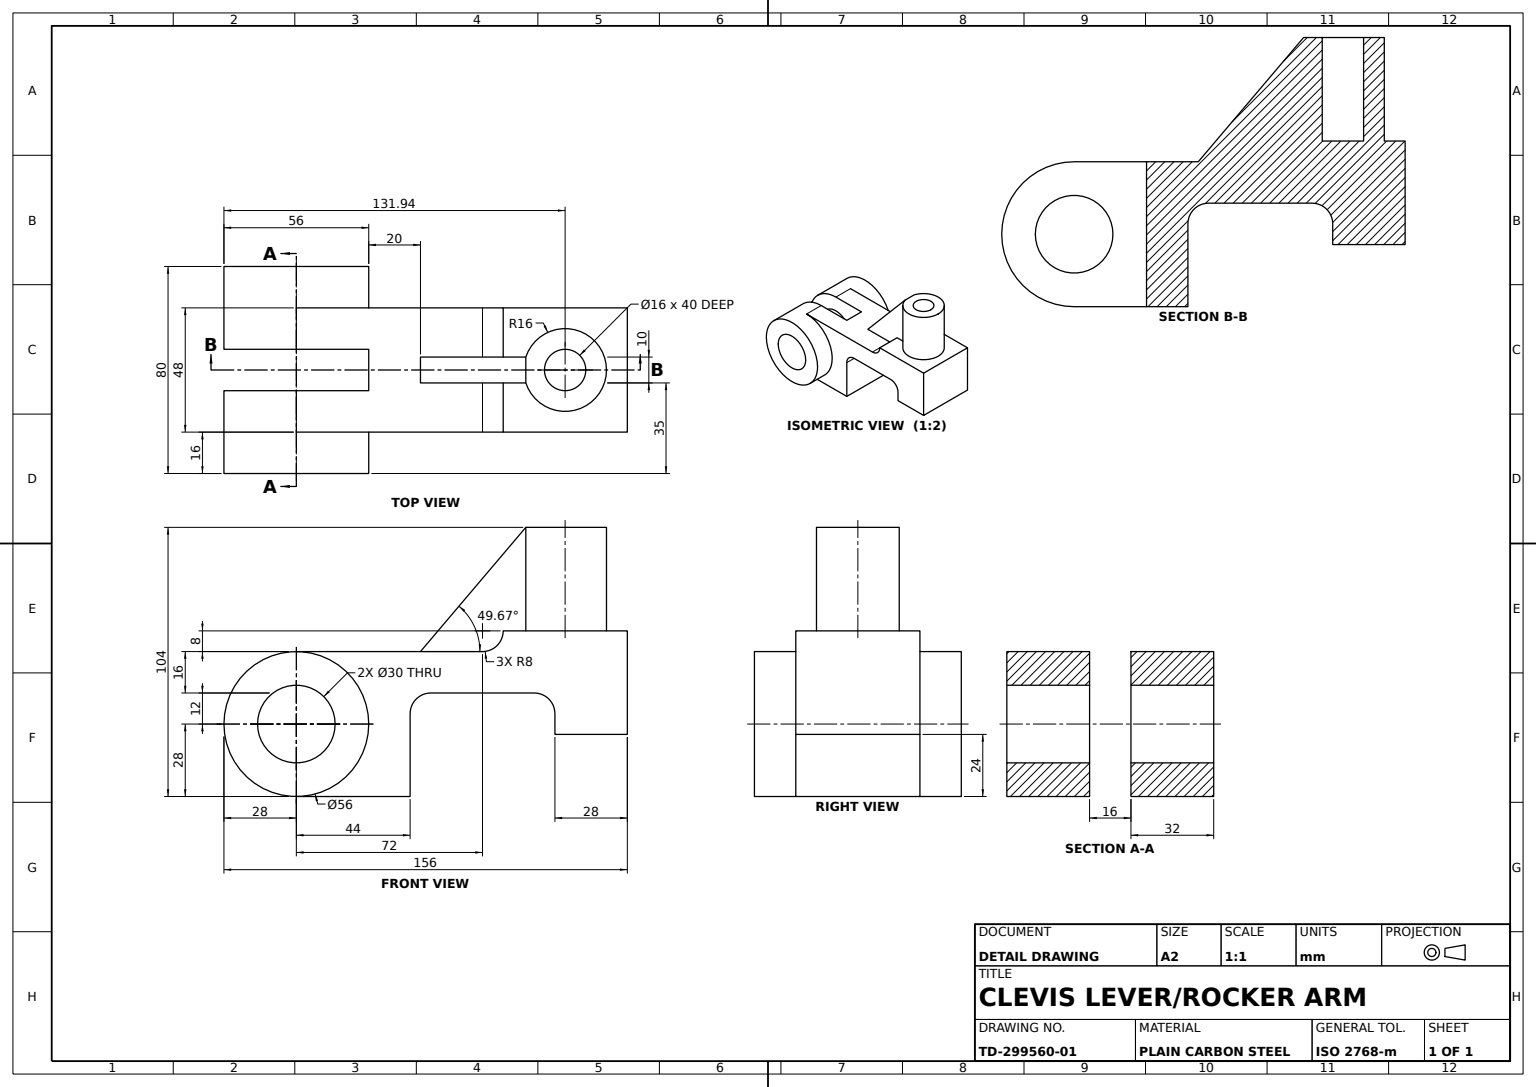
from build123d import *

# Parameters (mm, degrees)
PIVOT_HUB_SKETCH_R            = 28
PIVOT_HUB_SKETCH_R_2          = 15
PIVOT_HUB_56_BORE_30_DEPTH    = 40
LINK_ARM_DEPTH                = 24
FORK_SLOT_SKETCH_W            = 63.247521784
FORK_SLOT_SKETCH_H            = 16
FORK_SLOT_16_DEPTH            = 146.327216997
UPRIGHT_BOSS_SKETCH_R         = 16
UPRIGHT_BOSS_SKETCH_R_2       = 8
UPRIGHT_BOSS_32_BORE_16_DEPTH = 40
JUNCTION_PAD_REACH            = 171.706
TRIANGULAR_RELIEF_CUT_DEPTH   = 10


with BuildPart() as part:
    # Pivot Hub Sketch → Pivot Hub Ø56 Bore Ø30 (new, symmetric)
    with BuildSketch(Plane.XY):
        Circle(PIVOT_HUB_SKETCH_R)
        Circle(PIVOT_HUB_SKETCH_R_2, mode=Mode.SUBTRACT)
    extrude(amount=PIVOT_HUB_56_BORE_30_DEPTH, both=True)

    # Link Arm Profile → Link Arm (add, symmetric)
    with BuildSketch(Plane.XY):
        with BuildLine():
            Line((0, 28), (72, 28))
            ThreePointArc((72, 28), (77.656854249, 30.343145751), (80, 36))
            Line((80, 36), (128, 36))
            Line((128, 36), (128, -4))
            Line((128, -4), (100, -4))
            Line((100, -4), (100, 4))
            ThreePointArc((100, 4), (97.656854249, 9.656854249), (92, 12))
            Line((92, 12), (52, 12))
            ThreePointArc((52, 12), (46.343145751, 9.656854249), (44, 4))
            Line((44, 4), (44, -28))
            Line((44, -28), (0, -28))
            ThreePointArc((0, -28), (28, 0), (0, 28))
        make_face()
    extrude(amount=LINK_ARM_DEPTH, both=True)

    # Fork Slot Sketch → Fork Slot 16 (cut, through all)
    with BuildSketch(Plane(origin=(0, 28, 0), x_dir=(1, 0, 0), z_dir=(0, 1, 0))):
        with Locations((-3.623760892, 0)):
            Rectangle(FORK_SLOT_SKETCH_W, FORK_SLOT_SKETCH_H)
    extrude(amount=-FORK_SLOT_16_DEPTH, mode=Mode.SUBTRACT)

    # Upright Boss Sketch → Upright Boss Ø32 Bore Ø16 (add)
    with BuildSketch(Plane(origin=(0, 36, 0), x_dir=(1, 0, 0), z_dir=(0, 1, 0))):
        with Locations((103.942410132, 0)):
            Circle(UPRIGHT_BOSS_SKETCH_R)
        with Locations(Location((103.942410132, 0, 0), (0, 0, 180))):
            Circle(UPRIGHT_BOSS_SKETCH_R_2, mode=Mode.SUBTRACT)
    extrude(amount=UPRIGHT_BOSS_32_BORE_16_DEPTH)

    # Junction Pad Sketch → Junction Pad (add, up to next)
    with BuildSketch(Plane(origin=(0, 76, 0), x_dir=(1, 0, 0), z_dir=(0, 1, 0)), mode=Mode.PRIVATE) as junction_pad_sk1:
        with BuildLine():
            Line((48, 5), (88.743725978, 5))
            ThreePointArc((88.743725978, 5), (87.942410132, 0), (88.743725978, -5))
            Line((88.743725978, -5), (48, -5))
            Line((48, -5), (48, 5))
        make_face()
    junction_pad_tool1 = extrude(junction_pad_sk1.sketch, amount=-JUNCTION_PAD_REACH, mode=Mode.PRIVATE) - part.part
    add(junction_pad_tool1.solids().sort_by_distance((68.104095, 76, 0))[0])

    # Relief Cut Sketch → Triangular Relief Cut (cut)
    with BuildSketch(Plane.XY.offset(5)):
        Polygon((88.743725978, 76), (48, 28), (48, 76), align=None)
    extrude(amount=-TRIANGULAR_RELIEF_CUT_DEPTH, mode=Mode.SUBTRACT)


solid = part.part
